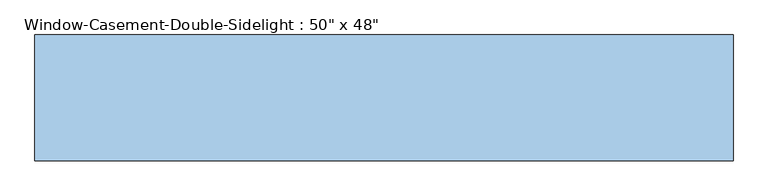
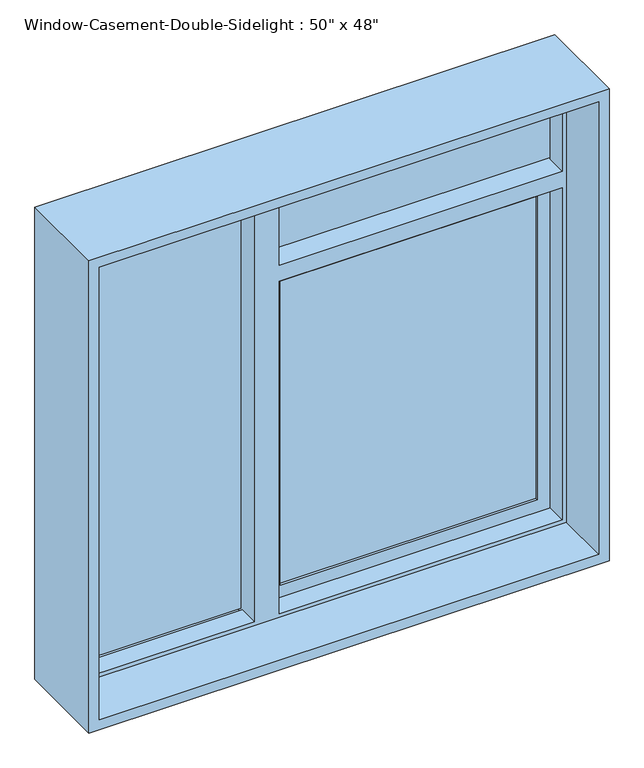
"""IFC4 building model written with IfcOpenShell, lengths in millimetres: window geometry."""

from ifc_helpers import new_model, si_unit, frame, origin, place, context, project, spatial, polyline, outline, extrude, faceted_brep, source, transform, mapped, element, save


def window_ae1cb28a(model_context):
    return source(origin(), model_context, "Body", "SolidModel", [
        extrude(outline(polyline([(567.7296875, 98.425), (-59.7296875, 98.425), (-59.7296875, 111.125), (567.7296875, 111.125), (567.7296875, 98.425)])), frame((0.0, 0.0, 981.6703125), z_axis=(0.0, 0.0, 1.0), x_axis=(1.0, 0.0, 0.0)), (0.0, 0.0, 1.0), 784.3242187),
        extrude(outline(polyline([(567.7296875, 85.725), (567.7296875, 79.375), (-59.7296875, 79.375), (-59.7296875, 85.725), (567.7296875, 85.725)])), frame((0.0, 0.0, 981.6703125), z_axis=(0.0, 0.0, 1.0), x_axis=(1.0, 0.0, 0.0)), (0.0, 0.0, 1.0), 784.3242187),
        extrude(outline(polyline([(-152.4, 98.425), (-152.4, 92.075), (-609.6, 92.075), (-609.6, 98.425), (-152.4, 98.425)])), frame((0.0, 0.0, 949.9203125), z_axis=(0.0, 0.0, 1.0), x_axis=(1.0, 0.0, 0.0)), (0.0, 0.0, 1.0), 1158.2796875),
        extrude(outline(polyline([(-152.4, 85.725), (-152.4, 79.375), (-609.6, 79.375), (-609.6, 85.725), (-152.4, 85.725)])), frame((0.0, 0.0, 949.9203125), z_axis=(0.0, 0.0, 1.0), x_axis=(1.0, 0.0, 0.0)), (0.0, 0.0, 1.0), 1158.2796875),
        extrude(outline(polyline([(609.6, 85.725), (609.6, 79.375), (-101.6, 79.375), (-101.6, 85.725), (609.6, 85.725)])), frame((0.0, 0.0, 1849.7351563), z_axis=(0.0, 0.0, 1.0), x_axis=(1.0, 0.0, 0.0)), (0.0, 0.0, 1.0), 258.4648438),
        extrude(outline(polyline([(609.6, 98.425), (609.6, 92.075), (-101.6, 92.075), (-101.6, 98.425), (609.6, 98.425)])), frame((0.0, 0.0, 1849.7351563), z_axis=(0.0, 0.0, 1.0), x_axis=(1.0, 0.0, 0.0)), (0.0, 0.0, 1.0), 258.4648438),
        faceted_brep([(-609.6, 73.025, 2108.2), (-609.6, 114.3, 2108.2), (609.6, 114.3, 2108.2), (609.6, 73.025, 2108.2), (-101.6, 73.025, 2108.2), (-101.6, 111.125, 2108.2), (-152.4, 111.125, 2108.2), (-152.4, 73.025, 2108.2), (-599.4796875, 22.225, 2098.0796875), (-599.4796875, 73.025, 2098.0796875), (-152.4, 73.025, 2098.0796875), (-152.4, 22.225, 2098.0796875), (599.4796875, 73.025, 2098.0796875), (599.4796875, 22.225, 2098.0796875), (-91.4796875, 22.225, 2098.0796875), (-91.4796875, 73.025, 2098.0796875), (-609.6, -114.3, 2108.2), (-609.6, 22.225, 2108.2), (609.6, 22.225, 2108.2), (609.6, -114.3, 2108.2), (-635.0, 114.3, 2133.6), (-635.0, -114.3, 2133.6), (635.0, -114.3, 2133.6), (635.0, 114.3, 2133.6), (609.6, 114.3, 939.8), (609.6, 73.025, 939.8), (609.6, 73.025, 1807.8648438), (609.6, 111.125, 1807.8648438), (609.6, 111.125, 1849.7351563), (609.6, 73.025, 1849.7351563), (599.4796875, 73.025, 1849.7351563), (599.4796875, 22.225, 1849.7351563), (599.4796875, 73.025, 949.9203125), (599.4796875, 22.225, 949.9203125), (599.4796875, 22.225, 1807.8648438), (599.4796875, 73.025, 1807.8648438), (609.6, 22.225, 939.8), (609.6, -114.3, 939.8), (635.0, -114.3, 914.4), (635.0, 114.3, 914.4), (-609.6, 114.3, 939.8), (-609.6, 73.025, 939.8), (-152.4, 73.025, 939.8), (-152.4, 111.125, 939.8), (-101.6, 111.125, 939.8), (-101.6, 73.025, 939.8), (-91.4796875, 73.025, 949.9203125), (-91.4796875, 22.225, 949.9203125), (-599.4796875, 73.025, 949.9203125), (-599.4796875, 22.225, 949.9203125), (-152.4, 22.225, 949.9203125), (-152.4, 73.025, 949.9203125), (-609.6, 22.225, 939.8), (-609.6, -114.3, 939.8), (-635.0, -114.3, 914.4), (-635.0, 114.3, 914.4), (-91.4796875, 73.025, 1849.7351563), (-101.6, 73.025, 1849.7351563), (-101.6, 73.025, 1807.8648438), (-91.4796875, 73.025, 1807.8648438), (-91.4796875, 22.225, 1849.7351563), (-91.4796875, 22.225, 1807.8648438), (-101.6, 111.125, 1849.7351563), (-101.6, 111.125, 1807.8648438)], [[[0, 1, 2, 3, 4, 5, 6, 7]], [[8, 9, 10, 11]], [[12, 13, 14, 15]], [[16, 17, 18, 19]], [[20, 21, 22, 23]], [[3, 2, 24, 25, 26, 27, 28, 29]], [[13, 12, 30, 31]], [[32, 33, 34, 35]], [[19, 18, 36, 37]], [[23, 22, 38, 39]], [[25, 24, 40, 41, 42, 43, 44, 45]], [[33, 32, 46, 47]], [[48, 49, 50, 51]], [[37, 36, 52, 53]], [[39, 38, 54, 55]], [[1, 0, 41, 40]], [[12, 15, 56, 57, 4, 3, 29, 30]], [[46, 32, 35, 26, 25, 45, 58, 59]], [[41, 0, 7, 10, 9, 48, 51, 42]], [[9, 8, 49, 48]], [[17, 52, 36, 18], [13, 31, 60, 14], [33, 47, 61, 34], [49, 8, 11, 50]], [[17, 16, 53, 52]], [[22, 21, 54, 38], [16, 19, 37, 53]], [[21, 20, 55, 54]], [[20, 23, 39, 55], [2, 1, 40, 24]], [[43, 6, 5, 62, 28, 27, 63, 44]], [[6, 43, 42, 51, 50, 11, 10, 7]], [[15, 14, 60, 56]], [[47, 46, 59, 61]], [[5, 4, 57, 62]], [[45, 44, 63, 58]], [[63, 27, 26, 35, 34, 61, 59, 58]], [[28, 62, 57, 56, 60, 31, 30, 29]]]),
        extrude(outline(polyline([(1807.8648438, 609.6), (1807.8648438, -101.6), (939.8, -101.6), (939.8, 609.6), (1807.8648438, 609.6)]), holes=[polyline([(981.6703125, 567.7296875), (981.6703125, -59.7296875), (1765.9945313, -59.7296875), (1765.9945313, 567.7296875), (981.6703125, 567.7296875)])]), frame((0.0, 73.025, 0.0), z_axis=(0.0, 1.0, 0.0), x_axis=(0.0, 0.0, 1.0)), (0.0, 0.0, 1.0), 31.75),
    ])


if __name__ == "__main__":
    model = new_model("IFC4")
    model_context = context("Model", 3, world=origin())
    ifc_project = project(units=[si_unit("LENGTHUNIT", "METRE", prefix="MILLI")], contexts=[model_context])
    site = spatial("IfcSite", under=ifc_project)
    building = spatial("IfcBuilding", under=site)
    placement = place(None, origin())
    window_shape = window_ae1cb28a(model_context)
    element("IfcWindow", 1, ObjectType="Window-Casement-Double-Sidelight : 50\" x 48\"", at=placement, inside=building, context=model_context, shape_type="MappedRepresentation", body=[
        mapped(window_shape, transform((0.0, 0.0, 0.0), x_axis=(1.0, 0.0, 0.0), y_axis=(0.0, 1.0, 0.0), z_axis=(0.0, 0.0, 1.0))),
    ])
    save(model, "model.ifc")

# Revit data of these elements
# Type "Window-Casement-Double-Sidelight : 50\" x 48\""
#   Type Mark = "22"
#   Fire Rating = "0.5h"
#   Assembly Code = "B2020100"
#   Analytic Construction = "Double glazing - domestic"
#   Window Inset [instance default] = 0' - 0 5/8"
#   Wall Thickness [instance default] = 0' - 6"
#   Visual Light Transmittance = 0.81
#   Transom Height Ratio = 0.25
#   Transom Height = 1' - 0"
#   Thermal Resistance (R) = 1.8146 (h·ft²·°F)/BTU
#   Solar Heat Gain Coefficient = 0.76
#   Side Width = 1' - 8"
#   Rough Width = 4' - 2 1/2"
#   Rough Height = 4' - 0 1/2"
#   Opening Window Width = 2' - 6"
#   Opening Window Height = 3' - 0"
#   Heat Transfer Coefficient (U) = 0.5511 BTU/(h·ft²·°F)
#   Height = 4' - 0"
#   Frame Gap 3 [instance default] = 0' - 1 83/128"
#   Frame Gap 2 [instance default] = 0' - 0 5/8"
#   Frame Gap 1 = 0' - 1 51/128"
#   Default Sill Height = 3' - 0"
#   Width = 4' - 2"
#   Frame Material = Metal - Aluminum
#   Glass Panel Material = Glass
#   Wall Closure = (empty or 0)
# Element 1 (IfcWindow, "Window-Casement-Double-Sidelight : 50\" x 48\"")
#   Wall Thickness = 0' - 9"
#   Materials on its faces: "Metal - Aluminum", "Glass"
# Materials
#   "Metal - Aluminum": class "Metal", colour RGB 247 247 247, transparency 0
#   "Glass": class "Glass", colour RGB 0 128 192, transparency 0.75, Description = "Soda Lime Glass", Cost = 0
